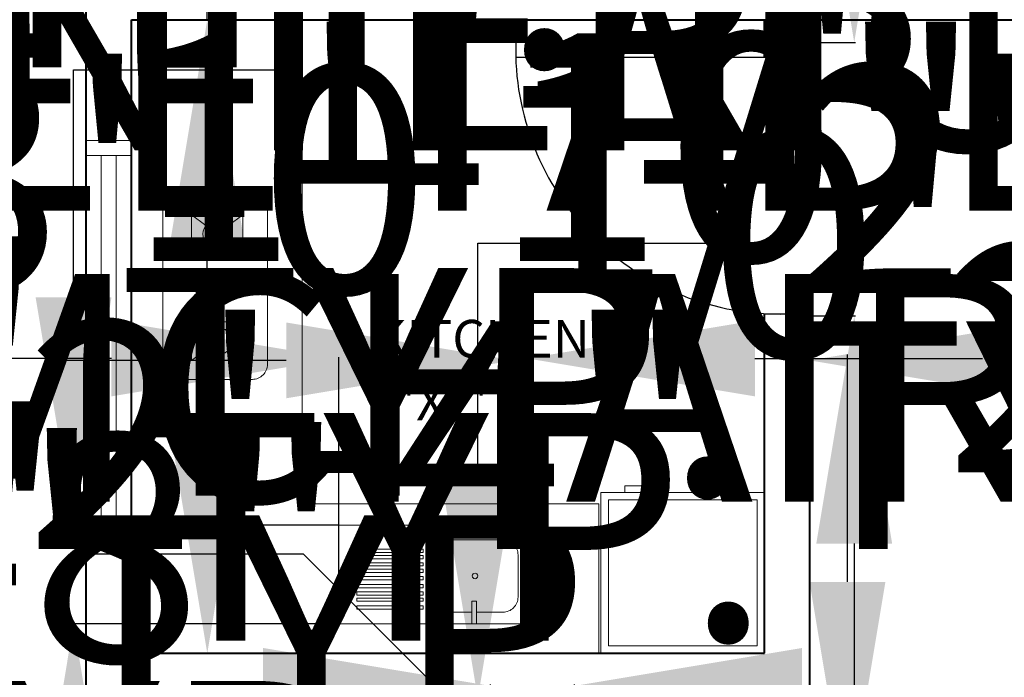
# Model space of a CAD drawing. Units: inches. Extents: x 7323 to 9737, y 2037 to 3322.
# Tile 10 of 19: x 8999 to 9130, y 2426 to 2513. Entities that reach past the tile are written whole.
import ezdxf

# ---------------------------------------------------------------- set-up
doc = ezdxf.new("R2010")
doc.units = ezdxf.units.IN
doc.header["$MEASUREMENT"] = 0
for name, color, linetype, lineweight in [('A-ANNO-DIMS', 2, 'Continuous', 18), ('A-AREA-IDEN', 7, 'Continuous', 18), ('A-DOOR', 4, 'Continuous', 25), ('A-EQPM', 9, 'Continuous', 18), ('A-FLOR-CASE', 9, 'Continuous', 20), ('A-FLOR-FIXT', 9, 'Continuous', 18), ('A-GLAZ', 4, 'Continuous', 18), ('A-WALL', 7, 'Continuous', 40)]:
    doc.layers.add(name, color=color, linetype=linetype, lineweight=lineweight)
doc.styles.get("Standard").update_dxf_attribs({"font": 'arial.ttf'})
doc.dimstyles.get("Standard").update_dxf_attribs({"dimtxt": 30.18, "dimasz": 30.18, "dimexe": 0.18, "dimexo": 0.0625, "dimgap": 0.09, "dimtad": 0, "dimtih": 1, "dimtoh": 1, "dimdec": 0, "dimzin": 0, "dimdsep": 46, "dimlunit": 3, "dimtxsty": 'Standard', "dimcen": 0.09, "dimadec": 0, "dimazin": 0, "dimtfac": 1, "dimtdec": 0, "dimtofl": 0, "dimtmove": 0, "dimatfit": 3, "dimfxl": 1, "dimtolj": 1, "dimtzin": 0, "dimarcsym": 0})

# ---------------------------------------------------------------- blocks, each defined once
blk = doc.blocks.new('*D11')
at = {"layer": 'A-ANNO-DIMS', "color": 0, "lineweight": -2, "transparency": 16777216}
for p, q in [((9007.88, 2687.3), (8985.8, 2687.3)), ((8985.98, 2657.12), (8985.98, 2458.79)), ((8985.98, 2229.48), (8985.98, 2427.8)), ((9007.88, 2199.3), (8985.8, 2199.3))]:
    blk.add_line(p, q, dxfattribs=at)
at = {"layer": 'A-ANNO-DIMS', "color": 0, "transparency": 16777216}
for points in [[(8980.95, 2657.12), (8991.01, 2657.12), (8985.98, 2687.3)], [(8980.95, 2229.48), (8991.01, 2229.48), (8985.98, 2199.3)]]:
    blk.add_solid(points, dxfattribs=at)
at = {"layer": 'Defpoints', "color": 0, "transparency": 16777216}
for p in [(9007.95, 2687.3), (8985.98, 2199.3), (9007.95, 2199.3)]:
    blk.add_point(p, dxfattribs=at)
at = {"layer": 'A-ANNO-DIMS', "color": 0, "transparency": 16777216, "insert": (8985.98, 2443.3), "char_height": 30.18, "attachment_point": 5}
blk.add_mtext('\\A1;40\'-8"', dxfattribs=at)
blk = doc.blocks.new('WIN-48')
for p, q in [((0, 0), (0, 6)), ((2, 0), (2, 6)), ((50, 0), (50, 6)), ((52, 0), (52, 6)), ((2, 4), (50, 4)), ((2, 2), (50, 2))]:
    blk.add_line(p, q)
blk = doc.blocks.new('DOOR-36-KITCHEN')
for p, q in [((33.01, 36.01), (0.01, 36.01)), ((36.01, 36.01), (39.01, 36.01)), ((36.01, 34.01), (36.01, 36.01)), ((36.01, 34.01), (0.01, 34.01)), ((33.01, 0.01), (39.01, 0.01))]:
    blk.add_line(p, q)
blk.add_arc((35.01, 35.01), 35.01, 178.3634, 271.6366)
blk = doc.blocks.new('KITCHEN-APPLIANCE')
for points in [[(21.71, 0), (21.71, 0), (0, 0), (0, 0), (0, 21.33), (0, 21.33), (21.71, 21.33), (21.71, 21.33)], [(3.16, 21.33), (3.16, 21.33), (7.58, 21.33), (7.58, 21.33), (7.58, 22.18), (7.58, 22.18), (3.16, 22.18), (3.16, 22.18)], [(20.71, 1), (1, 1), (1, 20.33), (20.71, 20.33)]]:
    blk.add_lwpolyline(points, close=True)
blk = doc.blocks.new('COUNTER-L')
for p, q in [((0, 84), (0, 19.81)), ((0, 19.81), (39.33, 19.81)), ((39.33, 19.81), (39.33, 0))]:
    blk.add_line(p, q)
blk = doc.blocks.new('*D39')
at = {"layer": 'A-ANNO-DIMS', "color": 0, "lineweight": -2, "transparency": 16777216}
for p, q in [((8647.94, 2549.03), (8617.76, 2549.03)), ((8678.12, 2543.2), (8678.12, 2549.21)), ((8717.39, 2543.2), (8717.39, 2549.21)), ((8747.57, 2549.03), (8777.75, 2549.03))]:
    blk.add_line(p, q, dxfattribs=at)
at = {"layer": 'A-ANNO-DIMS', "color": 0, "transparency": 16777216}
for points in [[(8647.94, 2554.06), (8647.94, 2544), (8678.12, 2549.03)], [(8747.57, 2554.06), (8747.57, 2544), (8717.39, 2549.03)]]:
    blk.add_solid(points, dxfattribs=at)
at = {"layer": 'Defpoints', "color": 0, "transparency": 16777216}
for p in [(8717.39, 2549.03), (8678.12, 2543.14), (8717.39, 2543.14)]:
    blk.add_point(p, dxfattribs=at)
at = {"layer": 'A-ANNO-DIMS', "color": 0, "transparency": 16777216, "insert": (9057.19, 2549.03), "char_height": 30.18, "attachment_point": 5}
blk.add_mtext('\\A1;SINGLE DOOR 3\'-3 1/2" TYP.', dxfattribs=at)
blk = doc.blocks.new('*D41')
at = {"layer": 'A-ANNO-DIMS', "color": 0, "lineweight": -2, "transparency": 16777216}
for p, q in [((8661.59, 2428.04), (8661.59, 2458.22)), ((8661.59, 2458.22), (8691.77, 2458.22)), ((8657.46, 2397.86), (8661.77, 2397.86)), ((8657.46, 2369.86), (8661.77, 2369.86)), ((8661.59, 2339.68), (8661.59, 2309.5))]:
    blk.add_line(p, q, dxfattribs=at)
at = {"layer": 'A-ANNO-DIMS', "color": 0, "transparency": 16777216}
for points in [[(8656.56, 2428.04), (8666.62, 2428.04), (8661.59, 2397.86)], [(8656.56, 2339.68), (8666.62, 2339.68), (8661.59, 2369.86)]]:
    blk.add_solid(points, dxfattribs=at)
at = {"layer": 'Defpoints', "color": 0, "transparency": 16777216}
for p in [(8657.39, 2397.86), (8661.59, 2397.86), (8657.39, 2369.86)]:
    blk.add_point(p, dxfattribs=at)
at = {"layer": 'A-ANNO-DIMS', "color": 0, "transparency": 16777216, "insert": (8945.06, 2458.22), "char_height": 30.18, "attachment_point": 5}
blk.add_mtext('\\A1;VENT WINDOW 2\'-4" TYP.', dxfattribs=at)
blk = doc.blocks.new('*D43')
at = {"layer": 'A-ANNO-DIMS', "color": 0, "lineweight": -2, "transparency": 16777216}
for p, q in [((9108.94, 2438.75), (9108.94, 2468.93)), ((9104.01, 2408.57), (9109.12, 2408.57)), ((9104.01, 2375.3), (9109.12, 2375.3)), ((9108.94, 2345.12), (9108.94, 2314.94))]:
    blk.add_line(p, q, dxfattribs=at)
at = {"layer": 'A-ANNO-DIMS', "color": 0, "transparency": 16777216}
for points in [[(9103.91, 2438.75), (9113.97, 2438.75), (9108.94, 2408.57)], [(9103.91, 2345.12), (9113.97, 2345.12), (9108.94, 2375.3)]]:
    blk.add_solid(points, dxfattribs=at)
at = {"layer": 'Defpoints', "color": 0, "transparency": 16777216}
for p in [(9103.95, 2408.57), (9108.94, 2408.57), (9103.95, 2375.3)]:
    blk.add_point(p, dxfattribs=at)
at = {"layer": 'A-ANNO-DIMS', "color": 0, "transparency": 16777216, "insert": (9108.94, 2391.93), "char_height": 30.18, "attachment_point": 5}
blk.add_mtext('\\A1;BATH DOOR 2\'-9 1/2" TYP.', dxfattribs=at)
blk = doc.blocks.new('*D44')
at = {"layer": 'A-ANNO-DIMS', "color": 0, "lineweight": -2, "transparency": 16777216}
for p, q in [((9070.67, 2375.23), (9070.67, 2370.12)), ((9103.95, 2375.23), (9103.95, 2370.12)), ((9040.49, 2370.3), (9010.31, 2370.3)), ((9134.13, 2370.3), (9164.31, 2370.3))]:
    blk.add_line(p, q, dxfattribs=at)
at = {"layer": 'A-ANNO-DIMS', "color": 0, "transparency": 16777216}
for points in [[(9040.49, 2375.33), (9040.49, 2365.27), (9070.67, 2370.3)], [(9134.13, 2375.33), (9134.13, 2365.27), (9103.95, 2370.3)]]:
    blk.add_solid(points, dxfattribs=at)
at = {"layer": 'Defpoints', "color": 0, "transparency": 16777216}
for p in [(9070.67, 2375.3), (9103.95, 2375.3), (9103.95, 2370.3)]:
    blk.add_point(p, dxfattribs=at)
at = {"layer": 'A-ANNO-DIMS', "color": 0, "transparency": 16777216, "insert": (9291.8, 2370.3), "char_height": 30.18, "attachment_point": 5}
blk.add_mtext('\\A1;2\'-9 1/2" TYP.', dxfattribs=at)
blk = doc.blocks.new('*D47')
at = {"layer": 'A-ANNO-DIMS', "color": 0, "lineweight": -2, "transparency": 16777216}
for p, q in [((8839.73, 2461.79), (8839.73, 2464.67)), ((8858.14, 2461.79), (8858.14, 2464.67)), ((8809.55, 2464.49), (8779.37, 2464.49)), ((8888.32, 2464.49), (8918.5, 2464.49))]:
    blk.add_line(p, q, dxfattribs=at)
at = {"layer": 'A-ANNO-DIMS', "color": 0, "transparency": 16777216}
for points in [[(8809.55, 2469.52), (8809.55, 2459.46), (8839.73, 2464.49)], [(8888.32, 2469.52), (8888.32, 2459.46), (8858.14, 2464.49)]]:
    blk.add_solid(points, dxfattribs=at)
at = {"layer": 'Defpoints', "color": 0, "transparency": 16777216}
for p in [(8858.14, 2464.49), (8839.73, 2461.73), (8858.14, 2461.73)]:
    blk.add_point(p, dxfattribs=at)
at = {"layer": 'A-ANNO-DIMS', "color": 0, "transparency": 16777216, "insert": (9164.9, 2464.49), "char_height": 30.18, "attachment_point": 5}
blk.add_mtext('\\A1;ARMCHAIR 1\'-6 1/2" TYP.', dxfattribs=at)
blk = doc.blocks.new('*D48')
at = {"layer": 'A-ANNO-DIMS', "color": 0, "lineweight": -2, "transparency": 16777216}
for p, q in [((8836.96, 2491.91), (8836.96, 2522.09)), ((8836.96, 2522.09), (8867.14, 2522.09)), ((8839.66, 2461.73), (8836.78, 2461.73)), ((8839.66, 2451.75), (8836.78, 2451.75)), ((8836.96, 2421.57), (8836.96, 2391.39))]:
    blk.add_line(p, q, dxfattribs=at)
at = {"layer": 'A-ANNO-DIMS', "color": 0, "transparency": 16777216}
for points in [[(8831.93, 2491.91), (8841.99, 2491.91), (8836.96, 2461.73)], [(8831.93, 2421.57), (8841.99, 2421.57), (8836.96, 2451.75)]]:
    blk.add_solid(points, dxfattribs=at)
at = {"layer": 'Defpoints', "color": 0, "transparency": 16777216}
for p in [(8836.96, 2461.73), (8839.73, 2461.73), (8839.73, 2451.75)]:
    blk.add_point(p, dxfattribs=at)
at = {"layer": 'A-ANNO-DIMS', "color": 0, "transparency": 16777216, "insert": (8970.94, 2522.09), "char_height": 30.18, "attachment_point": 5}
blk.add_mtext('\\A1;0\'-10" TYP.', dxfattribs=at)
blk = doc.blocks.new('*D52')
at = {"layer": 'A-ANNO-DIMS', "color": 0, "lineweight": -2, "transparency": 16777216}
for p, q in [((9220.65, 2583.03), (9220.65, 2613.21)), ((9209.01, 2552.85), (9220.83, 2552.85)), ((9209.01, 2513.3), (9220.83, 2513.3)), ((9220.65, 2483.12), (9220.65, 2452.94))]:
    blk.add_line(p, q, dxfattribs=at)
at = {"layer": 'A-ANNO-DIMS', "color": 0, "transparency": 16777216}
for points in [[(9215.62, 2583.03), (9225.68, 2583.03), (9220.65, 2552.85)], [(9215.62, 2483.12), (9225.68, 2483.12), (9220.65, 2513.3)]]:
    blk.add_solid(points, dxfattribs=at)
at = {"layer": 'Defpoints', "color": 0, "transparency": 16777216}
for p in [(9208.95, 2552.85), (9220.65, 2552.85), (9208.95, 2513.3)]:
    blk.add_point(p, dxfattribs=at)
at = {"layer": 'A-ANNO-DIMS', "color": 0, "transparency": 16777216, "insert": (9220.65, 2533.07), "char_height": 30.18, "attachment_point": 5}
blk.add_mtext('\\A1;3\'-3 1/2" TYP.', dxfattribs=at)
blk = doc.blocks.new('*D53')
at = {"layer": 'A-ANNO-DIMS', "color": 0, "lineweight": -2, "transparency": 16777216}
for p, q in [((8826.85, 2511.06), (8796.67, 2511.06)), ((8857.03, 2503.93), (8857.03, 2511.24)), ((8905.03, 2503.93), (8905.03, 2511.24)), ((8935.21, 2511.06), (8965.39, 2511.06))]:
    blk.add_line(p, q, dxfattribs=at)
at = {"layer": 'A-ANNO-DIMS', "color": 0, "transparency": 16777216}
for points in [[(8826.85, 2516.09), (8826.85, 2506.03), (8857.03, 2511.06)], [(8935.21, 2516.09), (8935.21, 2506.03), (8905.03, 2511.06)]]:
    blk.add_solid(points, dxfattribs=at)
at = {"layer": 'Defpoints', "color": 0, "transparency": 16777216}
for p in [(8905.03, 2511.06), (8857.03, 2503.86), (8905.03, 2503.86)]:
    blk.add_point(p, dxfattribs=at)
at = {"layer": 'A-ANNO-DIMS', "color": 0, "transparency": 16777216, "insert": (9261.3, 2511.06), "char_height": 30.18, "attachment_point": 5}
blk.add_mtext('\\A1;INTERIOR WINDOW 4\'-0" TYP.', dxfattribs=at)
blk = doc.blocks.new('*D54')
at = {"layer": 'A-ANNO-DIMS', "color": 0, "lineweight": -2, "transparency": 16777216}
for p, q in [((8849.83, 2534.04), (8849.83, 2564.22)), ((8849.83, 2564.22), (8880.01, 2564.22)), ((8856.96, 2503.86), (8849.65, 2503.86)), ((8856.96, 2497.86), (8849.65, 2497.86)), ((8849.83, 2467.68), (8849.83, 2437.5))]:
    blk.add_line(p, q, dxfattribs=at)
at = {"layer": 'A-ANNO-DIMS', "color": 0, "transparency": 16777216}
for points in [[(8844.8, 2534.04), (8854.86, 2534.04), (8849.83, 2503.86)], [(8844.8, 2467.68), (8854.86, 2467.68), (8849.83, 2497.86)]]:
    blk.add_solid(points, dxfattribs=at)
at = {"layer": 'Defpoints', "color": 0, "transparency": 16777216}
for p in [(8849.83, 2503.86), (8857.03, 2503.86), (8857.03, 2497.86)]:
    blk.add_point(p, dxfattribs=at)
at = {"layer": 'A-ANNO-DIMS', "color": 0, "transparency": 16777216, "insert": (8972.08, 2564.22), "char_height": 30.18, "attachment_point": 5}
blk.add_mtext('\\A1;0\'-6" TYP.', dxfattribs=at)
blk = doc.blocks.new('*D59')
at = {"layer": 'A-ANNO-DIMS', "color": 0, "lineweight": -2, "transparency": 16777216}
for p, q in [((9064.67, 2473.96), (9064.67, 2467.95)), ((9103.95, 2473.96), (9103.95, 2467.95)), ((9034.49, 2468.13), (9004.31, 2468.13)), ((9134.13, 2468.13), (9164.31, 2468.13))]:
    blk.add_line(p, q, dxfattribs=at)
at = {"layer": 'A-ANNO-DIMS', "color": 0, "transparency": 16777216}
for points in [[(9034.49, 2473.16), (9034.49, 2463.1), (9064.67, 2468.13)], [(9134.13, 2473.16), (9134.13, 2463.1), (9103.95, 2468.13)]]:
    blk.add_solid(points, dxfattribs=at)
at = {"layer": 'Defpoints', "color": 0, "transparency": 16777216}
for p in [(9064.67, 2474.02), (9103.95, 2474.02), (9103.95, 2468.13)]:
    blk.add_point(p, dxfattribs=at)
at = {"layer": 'A-ANNO-DIMS', "color": 0, "transparency": 16777216, "insert": (9458.35, 2468.13), "char_height": 30.18, "attachment_point": 5}
blk.add_mtext('\\A1;KITCHEN DOOR 3\'-3 1/2" TYP.', dxfattribs=at)
blk = doc.blocks.new('*D60')
at = {"layer": 'A-ANNO-DIMS', "color": 0, "lineweight": -2, "transparency": 16777216}
for p, q in [((9109.84, 2540.48), (9109.84, 2570.66)), ((9104.01, 2510.3), (9110.02, 2510.3)), ((9104.01, 2474.02), (9110.02, 2474.02)), ((9109.84, 2443.84), (9109.84, 2413.66))]:
    blk.add_line(p, q, dxfattribs=at)
at = {"layer": 'A-ANNO-DIMS', "color": 0, "transparency": 16777216}
for points in [[(9104.81, 2540.48), (9114.87, 2540.48), (9109.84, 2510.3)], [(9104.81, 2443.84), (9114.87, 2443.84), (9109.84, 2474.02)]]:
    blk.add_solid(points, dxfattribs=at)
at = {"layer": 'Defpoints', "color": 0, "transparency": 16777216}
for p in [(9103.95, 2510.3), (9109.84, 2510.3), (9103.95, 2474.02)]:
    blk.add_point(p, dxfattribs=at)
at = {"layer": 'A-ANNO-DIMS', "color": 0, "transparency": 16777216, "insert": (9109.84, 2492.16), "char_height": 30.18, "attachment_point": 5}
blk.add_mtext('\\A1;3\'-0 1/2" TYP.', dxfattribs=at)
blk = doc.blocks.new('*D63')
at = {"layer": 'A-ANNO-DIMS', "color": 0, "lineweight": -2, "transparency": 16777216}
for p, q in [((8744.72, 2466.22), (8744.72, 2496.4)), ((8744.72, 2496.4), (8774.9, 2496.4)), ((8741.46, 2436.04), (8744.9, 2436.04)), ((8741.46, 2413.86), (8744.9, 2413.86)), ((8744.72, 2383.68), (8744.72, 2353.5))]:
    blk.add_line(p, q, dxfattribs=at)
at = {"layer": 'A-ANNO-DIMS', "color": 0, "transparency": 16777216}
for points in [[(8739.69, 2466.22), (8749.75, 2466.22), (8744.72, 2436.04)], [(8739.69, 2383.68), (8749.75, 2383.68), (8744.72, 2413.86)]]:
    blk.add_solid(points, dxfattribs=at)
at = {"layer": 'Defpoints', "color": 0, "transparency": 16777216}
for p in [(8741.39, 2436.04), (8744.72, 2436.04), (8741.39, 2413.86)]:
    blk.add_point(p, dxfattribs=at)
at = {"layer": 'A-ANNO-DIMS', "color": 0, "transparency": 16777216, "insert": (9003.76, 2496.4), "char_height": 30.18, "attachment_point": 5}
blk.add_mtext('\\A1;APPLIANCE 1\'-10" TYP.', dxfattribs=at)
blk = doc.blocks.new('*D64')
at = {"layer": 'A-ANNO-DIMS', "color": 0, "lineweight": -2, "transparency": 16777216}
for p, q in [((8719.69, 2413.8), (8719.69, 2410.36)), ((8741.39, 2413.8), (8741.39, 2410.36)), ((8689.51, 2410.54), (8659.33, 2410.54)), ((8771.57, 2410.54), (8801.75, 2410.54))]:
    blk.add_line(p, q, dxfattribs=at)
at = {"layer": 'A-ANNO-DIMS', "color": 0, "transparency": 16777216}
for points in [[(8689.51, 2415.57), (8689.51, 2405.51), (8719.69, 2410.54)], [(8771.57, 2415.57), (8771.57, 2405.51), (8741.39, 2410.54)]]:
    blk.add_solid(points, dxfattribs=at)
at = {"layer": 'Defpoints', "color": 0, "transparency": 16777216}
for p in [(8719.69, 2413.86), (8741.39, 2413.86), (8741.39, 2410.54)]:
    blk.add_point(p, dxfattribs=at)
at = {"layer": 'A-ANNO-DIMS', "color": 0, "transparency": 16777216, "insert": (8927.57, 2410.54), "char_height": 30.18, "attachment_point": 5}
blk.add_mtext('\\A1;1\'-9 1/2" TYP.', dxfattribs=at)
blk = doc.blocks.new('*D65')
at = {"layer": 'A-ANNO-DIMS', "color": 0, "lineweight": -2, "transparency": 16777216}
for p, q in [((9024.02, 2513.3), (9024.02, 2543.48)), ((9024.02, 2543.48), (9054.2, 2543.48)), ((9036.56, 2513.3), (9023.84, 2513.3)), ((9024.02, 2459.48), (9024.02, 2483.12)), ((9036.56, 2429.3), (9023.84, 2429.3))]:
    blk.add_line(p, q, dxfattribs=at)
at = {"layer": 'A-ANNO-DIMS', "color": 0, "transparency": 16777216}
for points in [[(9018.99, 2483.12), (9029.05, 2483.12), (9024.02, 2513.3)], [(9018.99, 2459.48), (9029.05, 2459.48), (9024.02, 2429.3)]]:
    blk.add_solid(points, dxfattribs=at)
at = {"layer": 'Defpoints', "color": 0, "transparency": 16777216}
for p in [(9024.02, 2513.3), (9036.62, 2513.3), (9036.62, 2429.3)]:
    blk.add_point(p, dxfattribs=at)
at = {"layer": 'A-ANNO-DIMS', "color": 0, "transparency": 16777216, "insert": (9256.18, 2543.48), "char_height": 30.18, "attachment_point": 5}
blk.add_mtext('\\A1;COUNTER 7\'-0" TYP.', dxfattribs=at)
blk = doc.blocks.new('*D66')
at = {"layer": 'A-ANNO-DIMS', "color": 0, "lineweight": -2, "transparency": 16777216}
for p, q in [((9036.62, 2513.36), (9036.62, 2526.08)), ((9075.95, 2513.36), (9075.95, 2526.08)), ((9006.44, 2525.9), (8976.26, 2525.9)), ((9106.13, 2525.9), (9136.31, 2525.9))]:
    blk.add_line(p, q, dxfattribs=at)
at = {"layer": 'A-ANNO-DIMS', "color": 0, "transparency": 16777216}
for points in [[(9006.44, 2530.93), (9006.44, 2520.87), (9036.62, 2525.9)], [(9106.13, 2530.93), (9106.13, 2520.87), (9075.95, 2525.9)]]:
    blk.add_solid(points, dxfattribs=at)
at = {"layer": 'Defpoints', "color": 0, "transparency": 16777216}
for p in [(9075.95, 2525.9), (9036.62, 2513.3), (9075.95, 2513.3)]:
    blk.add_point(p, dxfattribs=at)
at = {"layer": 'A-ANNO-DIMS', "color": 0, "transparency": 16777216, "insert": (9263.53, 2525.9), "char_height": 30.18, "attachment_point": 5}
blk.add_mtext('\\A1;3\'-3 1/2" TYP.', dxfattribs=at)
blk = doc.blocks.new('*D69')
at = {"layer": 'A-ANNO-DIMS', "color": 0, "lineweight": -2, "transparency": 16777216}
for p, q in [((8836.58, 2472.89), (8836.58, 2503.07)), ((8836.58, 2503.07), (8866.76, 2503.07)), ((8839.88, 2442.71), (8836.4, 2442.71)), ((8839.88, 2420.33), (8836.4, 2420.33)), ((8836.58, 2390.15), (8836.58, 2359.97))]:
    blk.add_line(p, q, dxfattribs=at)
at = {"layer": 'A-ANNO-DIMS', "color": 0, "transparency": 16777216}
for points in [[(8831.55, 2472.89), (8841.61, 2472.89), (8836.58, 2442.71)], [(8831.55, 2390.15), (8841.61, 2390.15), (8836.58, 2420.33)]]:
    blk.add_solid(points, dxfattribs=at)
at = {"layer": 'Defpoints', "color": 0, "transparency": 16777216}
for p in [(8836.58, 2442.71), (8839.94, 2442.71), (8839.94, 2420.33)]:
    blk.add_point(p, dxfattribs=at)
at = {"layer": 'A-ANNO-DIMS', "color": 0, "transparency": 16777216, "insert": (9169.54, 2503.07), "char_height": 30.18, "attachment_point": 5}
blk.add_mtext('\\A1;COFFEE TABLE 1\'-10 1/2" TYP.', dxfattribs=at)
blk = doc.blocks.new('*D70')
at = {"layer": 'A-ANNO-DIMS', "color": 0, "lineweight": -2, "transparency": 16777216}
for p, q in [((8809.76, 2446.06), (8779.58, 2446.06)), ((8839.94, 2442.77), (8839.94, 2446.24)), ((8855.74, 2442.77), (8855.74, 2446.24)), ((8885.92, 2446.06), (8916.1, 2446.06))]:
    blk.add_line(p, q, dxfattribs=at)
at = {"layer": 'A-ANNO-DIMS', "color": 0, "transparency": 16777216}
for points in [[(8809.76, 2451.09), (8809.76, 2441.03), (8839.94, 2446.06)], [(8885.92, 2451.09), (8885.92, 2441.03), (8855.74, 2446.06)]]:
    blk.add_solid(points, dxfattribs=at)
at = {"layer": 'Defpoints', "color": 0, "transparency": 16777216}
for p in [(8855.74, 2446.06), (8839.94, 2442.71), (8855.74, 2442.71)]:
    blk.add_point(p, dxfattribs=at)
at = {"layer": 'A-ANNO-DIMS', "color": 0, "transparency": 16777216, "insert": (9006.75, 2446.06), "char_height": 30.18, "attachment_point": 5}
blk.add_mtext('\\A1;1\'-4" TYP.', dxfattribs=at)
blk = doc.blocks.new('*D71')
at = {"layer": 'A-ANNO-DIMS', "color": 0, "lineweight": -2, "transparency": 16777216}
for p, q in [((8891.18, 2486.02), (8891.18, 2516.2)), ((8884.24, 2455.84), (8891.36, 2455.84)), ((8884.24, 2409.18), (8891.36, 2409.18)), ((8891.18, 2379), (8891.18, 2348.82))]:
    blk.add_line(p, q, dxfattribs=at)
at = {"layer": 'A-ANNO-DIMS', "color": 0, "transparency": 16777216}
for points in [[(8886.15, 2486.02), (8896.21, 2486.02), (8891.18, 2455.84)], [(8886.15, 2379), (8896.21, 2379), (8891.18, 2409.18)]]:
    blk.add_solid(points, dxfattribs=at)
at = {"layer": 'Defpoints', "color": 0, "transparency": 16777216}
for p in [(8884.18, 2455.84), (8891.18, 2455.84), (8884.18, 2409.18)]:
    blk.add_point(p, dxfattribs=at)
at = {"layer": 'A-ANNO-DIMS', "color": 0, "transparency": 16777216, "insert": (8891.18, 2432.51), "char_height": 30.18, "attachment_point": 5}
blk.add_mtext('\\A1;SOFA 3\'-10 1/2" TYP.', dxfattribs=at)
blk = doc.blocks.new('*D72')
at = {"layer": 'A-ANNO-DIMS', "color": 0, "lineweight": -2, "transparency": 16777216}
for p, q in [((8864.06, 2409.12), (8864.06, 2402)), ((8884.18, 2409.12), (8884.18, 2402)), ((8833.88, 2402.18), (8803.7, 2402.18)), ((8914.36, 2402.18), (8944.54, 2402.18))]:
    blk.add_line(p, q, dxfattribs=at)
at = {"layer": 'A-ANNO-DIMS', "color": 0, "transparency": 16777216}
for points in [[(8833.88, 2407.21), (8833.88, 2397.15), (8864.06, 2402.18)], [(8914.36, 2407.21), (8914.36, 2397.15), (8884.18, 2402.18)]]:
    blk.add_solid(points, dxfattribs=at)
at = {"layer": 'Defpoints', "color": 0, "transparency": 16777216}
for p in [(8864.06, 2409.18), (8884.18, 2409.18), (8884.18, 2402.18)]:
    blk.add_point(p, dxfattribs=at)
at = {"layer": 'A-ANNO-DIMS', "color": 0, "transparency": 16777216, "insert": (9035.19, 2402.18), "char_height": 30.18, "attachment_point": 5}
blk.add_mtext('\\A1;1\'-8" TYP.', dxfattribs=at)
blk = doc.blocks.new('*D73')
at = {"layer": 'A-ANNO-DIMS', "color": 0, "lineweight": -2, "transparency": 16777216}
for p, q in [((9031.41, 2424.97), (9001.23, 2424.97)), ((9061.59, 2423.36), (9061.59, 2425.15)), ((9072.75, 2423.36), (9072.75, 2425.15)), ((9102.93, 2424.97), (9133.11, 2424.97))]:
    blk.add_line(p, q, dxfattribs=at)
at = {"layer": 'A-ANNO-DIMS', "color": 0, "transparency": 16777216}
for points in [[(9031.41, 2430), (9031.41, 2419.94), (9061.59, 2424.97)], [(9102.93, 2430), (9102.93, 2419.94), (9072.75, 2424.97)]]:
    blk.add_solid(points, dxfattribs=at)
at = {"layer": 'Defpoints', "color": 0, "transparency": 16777216}
for p in [(9072.75, 2424.97), (9061.59, 2423.3), (9072.75, 2423.3)]:
    blk.add_point(p, dxfattribs=at)
at = {"layer": 'A-ANNO-DIMS', "color": 0, "transparency": 16777216, "insert": (9305.36, 2424.97), "char_height": 30.18, "attachment_point": 5}
blk.add_mtext('\\A1;BASIN 0\'-11" TYP.', dxfattribs=at)
blk = doc.blocks.new('*D74')
at = {"layer": 'A-ANNO-DIMS', "color": 0, "lineweight": -2, "transparency": 16777216}
for p, q in [((9059.91, 2453.48), (9059.91, 2483.66)), ((9059.91, 2483.66), (9090.09, 2483.66)), ((9061.53, 2423.3), (9059.73, 2423.3)), ((9061.53, 2413.24), (9059.73, 2413.24)), ((9059.91, 2383.06), (9059.91, 2352.88))]:
    blk.add_line(p, q, dxfattribs=at)
at = {"layer": 'A-ANNO-DIMS', "color": 0, "transparency": 16777216}
for points in [[(9054.88, 2453.48), (9064.94, 2453.48), (9059.91, 2423.3)], [(9054.88, 2383.06), (9064.94, 2383.06), (9059.91, 2413.24)]]:
    blk.add_solid(points, dxfattribs=at)
at = {"layer": 'Defpoints', "color": 0, "transparency": 16777216}
for p in [(9059.91, 2423.3), (9061.59, 2423.3), (9061.59, 2413.24)]:
    blk.add_point(p, dxfattribs=at)
at = {"layer": 'A-ANNO-DIMS', "color": 0, "transparency": 16777216, "insert": (9193.89, 2483.66), "char_height": 30.18, "attachment_point": 5}
blk.add_mtext('\\A1;0\'-10" TYP.', dxfattribs=at)
blk = doc.blocks.new('*D79')
at = {"layer": 'A-ANNO-DIMS', "color": 0, "lineweight": -2, "transparency": 16777216}
for p, q in [((8871.1, 2395.97), (8871.1, 2394.46)), ((8880.36, 2395.97), (8880.36, 2394.46)), ((8840.92, 2394.64), (8810.74, 2394.64)), ((8910.54, 2394.64), (8940.72, 2394.64))]:
    blk.add_line(p, q, dxfattribs=at)
at = {"layer": 'A-ANNO-DIMS', "color": 0, "transparency": 16777216}
for points in [[(8840.92, 2399.67), (8840.92, 2389.61), (8871.1, 2394.64)], [(8910.54, 2399.67), (8910.54, 2389.61), (8880.36, 2394.64)]]:
    blk.add_solid(points, dxfattribs=at)
at = {"layer": 'Defpoints', "color": 0, "transparency": 16777216}
for p in [(8871.1, 2396.03), (8880.36, 2396.03), (8880.36, 2394.64)]:
    blk.add_point(p, dxfattribs=at)
at = {"layer": 'A-ANNO-DIMS', "color": 0, "transparency": 16777216, "insert": (9195.57, 2394.64), "char_height": 30.18, "attachment_point": 5}
blk.add_mtext('\\A1;SIDE TABLE 0\'-9 1/2" TYP.', dxfattribs=at)
blk = doc.blocks.new('*D80')
at = {"layer": 'A-ANNO-DIMS', "color": 0, "lineweight": -2, "transparency": 16777216}
for p, q in [((8881.74, 2435.12), (8881.74, 2465.3)), ((8881.74, 2465.3), (8911.92, 2465.3)), ((8880.42, 2404.94), (8881.92, 2404.94)), ((8880.42, 2396.03), (8881.92, 2396.03)), ((8881.74, 2365.85), (8881.74, 2335.67))]:
    blk.add_line(p, q, dxfattribs=at)
at = {"layer": 'A-ANNO-DIMS', "color": 0, "transparency": 16777216}
for points in [[(8876.71, 2435.12), (8886.77, 2435.12), (8881.74, 2404.94)], [(8876.71, 2365.85), (8886.77, 2365.85), (8881.74, 2396.03)]]:
    blk.add_solid(points, dxfattribs=at)
at = {"layer": 'Defpoints', "color": 0, "transparency": 16777216}
for p in [(8880.36, 2404.94), (8881.74, 2404.94), (8880.36, 2396.03)]:
    blk.add_point(p, dxfattribs=at)
at = {"layer": 'A-ANNO-DIMS', "color": 0, "transparency": 16777216, "insert": (9003.99, 2465.3), "char_height": 30.18, "attachment_point": 5}
blk.add_mtext('\\A1;0\'-9" TYP.', dxfattribs=at)
blk = doc.blocks.new('*D106')
at = {"layer": 'A-ANNO-DIMS', "color": 0, "lineweight": -2, "transparency": 16777216}
for p, q in [((9008.12, 2519.31), (8587.16, 2519.31)), ((8587.34, 2489.13), (8587.34, 2439.14)), ((8587.34, 2357.76), (8587.34, 2407.75)), ((9008.23, 2327.58), (8587.16, 2327.58))]:
    blk.add_line(p, q, dxfattribs=at)
at = {"layer": 'A-ANNO-DIMS', "color": 0, "transparency": 16777216}
for points in [[(8582.31, 2489.13), (8592.37, 2489.13), (8587.34, 2519.31)], [(8582.31, 2357.76), (8592.37, 2357.76), (8587.34, 2327.58)]]:
    blk.add_solid(points, dxfattribs=at)
at = {"layer": 'Defpoints', "color": 0, "transparency": 16777216}
for p in [(8587.34, 2519.31), (9008.18, 2519.31), (9008.29, 2327.58)]:
    blk.add_point(p, dxfattribs=at)
at = {"layer": 'A-ANNO-DIMS', "color": 0, "transparency": 16777216, "insert": (8587.34, 2423.44), "char_height": 30.18, "attachment_point": 5}
blk.add_mtext('\\A1;15\'-11 1/2"', dxfattribs=at)
blk = doc.blocks.new('*D110')
at = {"layer": 'A-ANNO-DIMS', "color": 0, "lineweight": -2, "transparency": 16777216}
for p, q in [((8587.34, 2449.91), (8587.34, 2480.09)), ((9018.85, 2419.73), (8587.16, 2419.73)), ((9018.85, 2375.3), (8587.16, 2375.3)), ((8587.34, 2345.12), (8587.34, 2314.94))]:
    blk.add_line(p, q, dxfattribs=at)
at = {"layer": 'A-ANNO-DIMS', "color": 0, "transparency": 16777216}
for points in [[(8582.31, 2449.91), (8592.37, 2449.91), (8587.34, 2419.73)], [(8582.31, 2345.12), (8592.37, 2345.12), (8587.34, 2375.3)]]:
    blk.add_solid(points, dxfattribs=at)
at = {"layer": 'Defpoints', "color": 0, "transparency": 16777216}
for p in [(8587.34, 2419.73), (9018.91, 2419.73), (9018.91, 2375.3)]:
    blk.add_point(p, dxfattribs=at)
at = {"layer": 'A-ANNO-DIMS', "color": 0, "transparency": 16777216, "insert": (8587.34, 2397.51), "char_height": 30.18, "attachment_point": 5}
blk.add_mtext('\\A1;3\'-8 1/2"', dxfattribs=at)
blk = doc.blocks.new('*D111')
at = {"layer": 'A-ANNO-DIMS', "color": 0, "lineweight": -2, "transparency": 16777216}
for p, q in [((9041.479226, 2433.251449), (9041.479226, 2468.568949)), ((9066.478924, 2433.251449), (9066.478924, 2468.568949)), ((9011.299226, 2468.388949), (8981.119226, 2468.388949)), ((9096.658924, 2468.388949), (9126.838924, 2468.388949))]:
    blk.add_line(p, q, dxfattribs=at)
at = {"layer": 'A-ANNO-DIMS', "color": 0, "transparency": 16777216}
for points in [[(9011.299226, 2473.418949), (9011.299226, 2463.358949), (9041.479226, 2468.388949)], [(9096.658924, 2473.418949), (9096.658924, 2463.358949), (9066.478924, 2468.388949)]]:
    blk.add_solid(points, dxfattribs=at)
at = {"layer": 'Defpoints', "color": 0, "transparency": 16777216}
for p in [(9066.478924, 2468.388949), (9041.479226, 2433.188949), (9066.478924, 2433.188949)]:
    blk.add_point(p, dxfattribs=at)
at = {"layer": 'A-ANNO-DIMS', "color": 0, "transparency": 16777216, "insert": (9167.299306, 2468.388949), "char_height": 30.18, "attachment_point": 5}
blk.add_mtext('\\A1;2\'-1"', dxfattribs=at)
blk = doc.blocks.new('*D112')
at = {"layer": 'A-ANNO-DIMS', "color": 0, "lineweight": -2, "transparency": 16777216}
for p, q in [((9006.28, 2476.47), (9006.28, 2506.65)), ((9006.28, 2506.65), (9036.46, 2506.65)), ((9041.42, 2446.29), (9006.1, 2446.29)), ((9041.42, 2433.19), (9006.1, 2433.19)), ((9006.28, 2403.01), (9006.28, 2372.83))]:
    blk.add_line(p, q, dxfattribs=at)
at = {"layer": 'A-ANNO-DIMS', "color": 0, "transparency": 16777216}
for points in [[(9001.25, 2476.47), (9011.31, 2476.47), (9006.28, 2446.29)], [(9001.25, 2403.01), (9011.31, 2403.01), (9006.28, 2433.19)]]:
    blk.add_solid(points, dxfattribs=at)
at = {"layer": 'Defpoints', "color": 0, "transparency": 16777216}
for p in [(9006.28, 2446.29), (9041.48, 2446.29), (9041.48, 2433.19)]:
    blk.add_point(p, dxfattribs=at)
at = {"layer": 'A-ANNO-DIMS', "color": 0, "transparency": 16777216, "insert": (9075.24, 2506.65), "char_height": 30.18, "attachment_point": 5}
blk.add_mtext('\\A1;1\'-1"', dxfattribs=at)
blk = doc.blocks.new('*D127')
at = {"layer": 'A-ANNO-DIMS', "color": 0, "lineweight": -2, "transparency": 16777216}
for p, q in [((9006.57, 2442.49), (9036.75, 2442.49)), ((9036.75, 2442.49), (9058.09, 2421.15)), ((9099.86, 2379.3), (9100.04, 2379.3)), ((9099.95, 2379.21), (9099.95, 2379.39))]:
    blk.add_line(p, q, dxfattribs=at)
at = {"layer": 'A-ANNO-DIMS', "color": 0, "transparency": 16777216}
blk.add_solid([(9061.64, 2424.71), (9054.53, 2417.6), (9079.43, 2399.81)], dxfattribs=at)
at = {"layer": 'Defpoints', "color": 0, "transparency": 16777216}
for p in [(9079.43, 2399.81), (9099.95, 2379.3)]:
    blk.add_point(p, dxfattribs=at)
at = {"layer": 'A-ANNO-DIMS', "color": 0, "transparency": 16777216, "insert": (8951.92, 2442.49), "char_height": 30.18, "attachment_point": 5}
blk.add_mtext('\\A1;R2\'-5"', dxfattribs=at)

msp = doc.modelspace()

# ---------------------------------------------------------------- linework, layer by layer
at = {"layer": 'A-EQPM'}
for p, q in [((9021.93, 2487.45), (9023.82, 2486.02)), ((9028.73, 2487.45), (9026.84, 2486.02)), ((9021.93, 2482.33), (9023.82, 2483.76)), ((9028.73, 2482.33), (9026.84, 2483.76)), ((9021.93, 2473.24), (9023.82, 2471.82)), ((9028.73, 2473.24), (9026.84, 2471.82)), ((9021.93, 2468.12), (9023.82, 2469.55)), ((9028.73, 2468.12), (9026.84, 2469.55))]:
    msp.add_line(p, q, dxfattribs=at)
msp.add_lwpolyline([(9018.12, 2487.92, -0.414214), (9020.12, 2489.92), (9030, 2489.92, -0.414214), (9032, 2487.92), (9032, 2467.61, -0.414214), (9030, 2465.61), (9020.12, 2465.61, -0.414214), (9018.12, 2467.61)], format="xyb", close=True, dxfattribs=at)
for points in [[(9021.93, 2487.45), (9021.93, 2487.45), (9028.73, 2487.45), (9028.73, 2487.45), (9028.73, 2482.33), (9028.73, 2482.33), (9021.93, 2482.33), (9021.93, 2482.33)], [(9021.93, 2473.24), (9021.93, 2473.24), (9028.73, 2473.24), (9028.73, 2473.24), (9028.73, 2468.12), (9028.73, 2468.12), (9021.93, 2468.12), (9021.93, 2468.12)]]:
    msp.add_lwpolyline(points, close=True, dxfattribs=at)
for centre in [(9025.33, 2484.89), (9025.33, 2470.68)]:
    msp.add_circle(centre, 1.89, dxfattribs=at)
at = {"layer": 'A-FLOR-FIXT'}
for points in [[(9041.48, 2446.29), (9041.48, 2446.29), (9066.48, 2446.29), (9066.48, 2446.29), (9066.48, 2433.19), (9066.48, 2433.19), (9041.48, 2433.19), (9041.48, 2433.19)], [(9043.84, 2443.09), (9043.84, 2443.09), (9052.65, 2443.09), (9052.65, 2443.09), (9052.65, 2442.66), (9052.65, 2442.66), (9043.84, 2442.66), (9043.84, 2442.66)], [(9043.84, 2442.25), (9043.84, 2442.25), (9052.65, 2442.25), (9052.65, 2442.25), (9052.65, 2441.81), (9052.65, 2441.81), (9043.84, 2441.81), (9043.84, 2441.81)], [(9043.84, 2441.3), (9043.84, 2441.3), (9052.65, 2441.3), (9052.65, 2441.3), (9052.65, 2440.87), (9052.65, 2440.87), (9043.84, 2440.87), (9043.84, 2440.87)], [(9043.84, 2440.45), (9043.84, 2440.45), (9052.65, 2440.45), (9052.65, 2440.45), (9052.65, 2440.02), (9052.65, 2440.02), (9043.84, 2440.02), (9043.84, 2440.02)], [(9043.84, 2439.47), (9043.84, 2439.47), (9052.65, 2439.47), (9052.65, 2439.47), (9052.65, 2439.04), (9052.65, 2439.04), (9043.84, 2439.04), (9043.84, 2439.04)], [(9043.84, 2438.42), (9043.84, 2438.42), (9052.65, 2438.42), (9052.65, 2438.42), (9052.65, 2437.98), (9052.65, 2437.98), (9043.84, 2437.98), (9043.84, 2437.98)], [(9043.84, 2437.43), (9043.84, 2437.43), (9052.65, 2437.43), (9052.65, 2437.43), (9052.65, 2437), (9052.65, 2437), (9043.84, 2437), (9043.84, 2437)], [(9043.84, 2436.62), (9043.84, 2436.62), (9052.65, 2436.62), (9052.65, 2436.62), (9052.65, 2436.19), (9052.65, 2436.19), (9043.84, 2436.19), (9043.84, 2436.19)], [(9059.75, 2433.19), (9059.75, 2433.19), (9059.13, 2433.19), (9059.13, 2433.19), (9059.13, 2436.21), (9059.13, 2436.21), (9059.75, 2436.21), (9059.75, 2436.21)], [(9043.84, 2435.57), (9043.84, 2435.57), (9052.65, 2435.57), (9052.65, 2435.57), (9052.65, 2435.14), (9052.65, 2435.14), (9043.84, 2435.14), (9043.84, 2435.14)]]:
    msp.add_lwpolyline(points, close=True, dxfattribs=at)
msp.add_lwpolyline([(9059.13, 2434.75), (9055.83, 2434.75, -0.414214), (9053.83, 2436.75), (9053.83, 2442.34, -0.414214), (9055.83, 2444.34), (9063.24, 2444.34, -0.414214), (9065.24, 2442.34), (9065.24, 2436.75, -0.414214), (9063.24, 2434.75), (9059.75, 2434.75)], format="xyb", dxfattribs=at)
msp.add_circle((9059.54, 2439.55), 0.364, dxfattribs=at)
at = {"layer": 'A-WALL'}
for p, q in [((9007.95, 2199.3), (9007.95, 2687.3)), ((9013.95, 2429.3), (9013.95, 2513.3)), ((9013.95, 2513.3), (9133.95, 2513.3)), ((9097.95, 2508.3), (9097.95, 2513.3)), ((9097.95, 2508.3), (9097.95, 2513.3)), ((9103.95, 2510.3), (9103.95, 2513.3)), ((9103.95, 2510.3), (9103.95, 2513.3)), ((9097.95, 2429.3), (9097.95, 2474.34)), ((9097.95, 2429.3), (9097.95, 2474.34)), ((9103.95, 2408.3), (9103.95, 2474.3)), ((9103.95, 2423.3), (9103.95, 2474.3)), ((9013.95, 2429.3), (9097.95, 2429.3))]:
    msp.add_line(p, q, dxfattribs=at)

# ---------------------------------------------------------------- block references
at = {"layer": 'A-DOOR'}
msp.add_blockref('DOOR-36-KITCHEN', (9064.93, 2474.28), dxfattribs=at)
at = {"layer": 'A-EQPM'}
msp.add_blockref('KITCHEN-APPLIANCE', (9076.24, 2429.3), dxfattribs=at)
at = {"layer": 'A-FLOR-CASE'}
msp.add_blockref('COUNTER-L', (9036.62, 2429.3), dxfattribs=at)
at = {"layer": 'A-GLAZ', "rotation": 89.99999999999586}
msp.add_blockref('WIN-48', (9013.95, 2445.3), dxfattribs=at)

# ---------------------------------------------------------------- texts
at = {"layer": 'A-AREA-IDEN', "insert": (9046.03, 2473.5), "char_height": 5, "attachment_point": 1}
msp.add_mtext_dynamic_manual_height_columns("KITCHEN\\P7'X7'", width=44.1759, gutter_width=1, heights=[0], dxfattribs=at)

# ---------------------------------------------------------------- dimensions: what is measured, and where the dimension line sits
at = {"layer": 'A-ANNO-DIMS'}
for base, p1, p2, override, picture, middle in [((8985.98, 2199.3), (9007.95, 2687.3), (9007.95, 2199.3), {"dimclrd": 0, "dimclre": 0, "dimclrt": 0}, '*D11', (8985.98, 2443.3)), ((9006.28, 2446.29), (9041.48, 2433.19), (9041.48, 2446.29), {"dimdec": 1, "dimlfac": 1, "dimrnd": 0, "dimzin": 1, "dimdsep": 46, "dimlunit": 4, "dimfrac": 2}, '*D112', (9075.24, 2506.65)), ((8587.34, 2519.31), (9008.29, 2327.58), (9008.18, 2519.31), {"dimdec": 1, "dimlfac": 1, "dimrnd": 0, "dimzin": 1, "dimdsep": 46, "dimlunit": 4, "dimfrac": 2}, '*D106', (8587.34, 2423.44)), ((8587.34, 2419.73), (9018.91, 2375.3), (9018.91, 2419.73), {"dimdec": 1, "dimlfac": 1, "dimrnd": 0, "dimzin": 1, "dimdsep": 46, "dimlunit": 4, "dimfrac": 2}, '*D110', (8587.34, 2397.51))]:
    dim = msp.add_linear_dim(base=base, p1=p1, p2=p2, angle=90, dimstyle='Standard', override=override, dxfattribs=at)
    dim.commit()
    dim.dimension.update_dxf_attribs({"geometry": picture, "text_midpoint": middle})
for base, p1, p2, text, picture, middle in [((8717.39, 2549.03), (8678.12, 2543.14), (8717.39, 2543.14), 'SINGLE DOOR <> TYP.', '*D39', (9057.19, 2549.03)), ((8905.03, 2511.06), (8857.03, 2503.86), (8905.03, 2503.86), 'INTERIOR WINDOW <> TYP.', '*D53', (9261.3, 2511.06)), ((9075.95, 2525.9), (9036.62, 2513.3), (9075.95, 2513.3), '<> TYP.', '*D66', (9263.53, 2525.9)), ((9103.95, 2468.13), (9064.67, 2474.02), (9103.95, 2474.02), 'KITCHEN DOOR <> TYP.', '*D59', (9458.35, 2468.13)), ((8858.14, 2464.49), (8839.73, 2461.73), (8858.14, 2461.73), 'ARMCHAIR <> TYP.', '*D47', (9164.9, 2464.49)), ((8880.36, 2394.64), (8871.1, 2396.03), (8880.36, 2396.03), 'SIDE TABLE <> TYP.', '*D79', (9195.57, 2394.64)), ((9072.75, 2424.97), (9061.59, 2423.3), (9072.75, 2423.3), 'BASIN <> TYP.', '*D73', (9305.36, 2424.97)), ((8855.74, 2446.06), (8839.94, 2442.71), (8855.74, 2442.71), '<> TYP.', '*D70', (9006.75, 2446.06)), ((8741.39, 2410.54), (8719.69, 2413.86), (8741.39, 2413.86), '<> TYP.', '*D64', (8927.57, 2410.54)), ((8884.18, 2402.18), (8864.06, 2409.18), (8884.18, 2409.18), '<> TYP.', '*D72', (9035.19, 2402.18)), ((9103.95, 2370.3), (9070.67, 2375.3), (9103.95, 2375.3), '<> TYP.', '*D44', (9291.8, 2370.3))]:
    dim = msp.add_linear_dim(base=base, p1=p1, p2=p2, text=text, dimstyle='Standard', override={"dimdec": 1, "dimlfac": 1, "dimrnd": 0, "dimzin": 1, "dimdsep": 46, "dimlunit": 4, "dimfrac": 2}, dxfattribs=at)
    dim.commit()
    dim.dimension.update_dxf_attribs({"geometry": picture, "text_midpoint": middle})
for base, p1, p2, text, picture, middle in [((8836.58, 2442.71), (8839.94, 2420.33), (8839.94, 2442.71), 'COFFEE TABLE <> TYP.', '*D69', (9169.54, 2503.07)), ((9024.02, 2513.3), (9036.62, 2429.3), (9036.62, 2513.3), 'COUNTER <> TYP.', '*D65', (9256.18, 2543.48)), ((9220.6454, 2552.8475), (9208.9454, 2513.2952), (9208.9454, 2552.8475), '<> TYP.', '*D52', (9220.6454, 2533.0713)), ((8849.83, 2503.86), (8857.03, 2497.86), (8857.03, 2503.86), '<> TYP.', '*D54', (8972.08, 2564.22)), ((9109.84, 2510.3), (9103.95, 2474.02), (9103.95, 2510.3), '<> TYP.', '*D60', (9109.84, 2492.16)), ((8744.72, 2436.04), (8741.39, 2413.86), (8741.39, 2436.04), 'APPLIANCE <> TYP.', '*D63', (9003.76, 2496.4)), ((8836.96, 2461.73), (8839.73, 2451.75), (8839.73, 2461.73), '<> TYP.', '*D48', (8970.94, 2522.09)), ((8661.59, 2397.86), (8657.39, 2369.86), (8657.39, 2397.86), 'VENT WINDOW <> TYP.', '*D41', (8945.06, 2458.22)), ((9059.91, 2423.3), (9061.59, 2413.24), (9061.59, 2423.3), '<> TYP.', '*D74', (9193.89, 2483.66)), ((8891.18, 2455.84), (8884.18, 2409.18), (8884.18, 2455.84), 'SOFA <> TYP.', '*D71', (8891.18, 2432.51)), ((9108.94, 2408.57), (9103.95, 2375.3), (9103.95, 2408.57), 'BATH DOOR <> TYP.', '*D43', (9108.94, 2391.93)), ((8881.74, 2404.94), (8880.36, 2396.03), (8880.36, 2404.94), '<> TYP.', '*D80', (9003.99, 2465.3))]:
    dim = msp.add_linear_dim(base=base, p1=p1, p2=p2, angle=90, text=text, dimstyle='Standard', override={"dimdec": 1, "dimlfac": 1, "dimrnd": 0, "dimzin": 1, "dimdsep": 46, "dimlunit": 4, "dimfrac": 2}, dxfattribs=at)
    dim.commit()
    dim.dimension.update_dxf_attribs({"geometry": picture, "text_midpoint": middle})
dim = msp.add_linear_dim(base=(9066.48, 2468.39), p1=(9041.48, 2433.19), p2=(9066.48, 2433.19), dimstyle='Standard', override={"dimdec": 1, "dimlfac": 1, "dimrnd": 0, "dimzin": 1, "dimdsep": 46, "dimlunit": 4, "dimfrac": 2}, dxfattribs=at)
dim.commit()
dim.dimension.update_dxf_attribs({"geometry": '*D111', "text_midpoint": (9167.3, 2468.39)})
dim = msp.add_radius_dim(center=(9099.95, 2379.3), mpoint=(9079.43, 2399.81), dimstyle='Standard', override={"dimdec": 1, "dimlfac": 1, "dimrnd": 0, "dimzin": 1, "dimdsep": 46, "dimlunit": 4, "dimfrac": 2}, dxfattribs=at)
dim.commit()
dim.dimension.update_dxf_attribs({"geometry": '*D127', "text_midpoint": (8951.92, 2442.49)})

doc.saveas('drawing.dxf')
